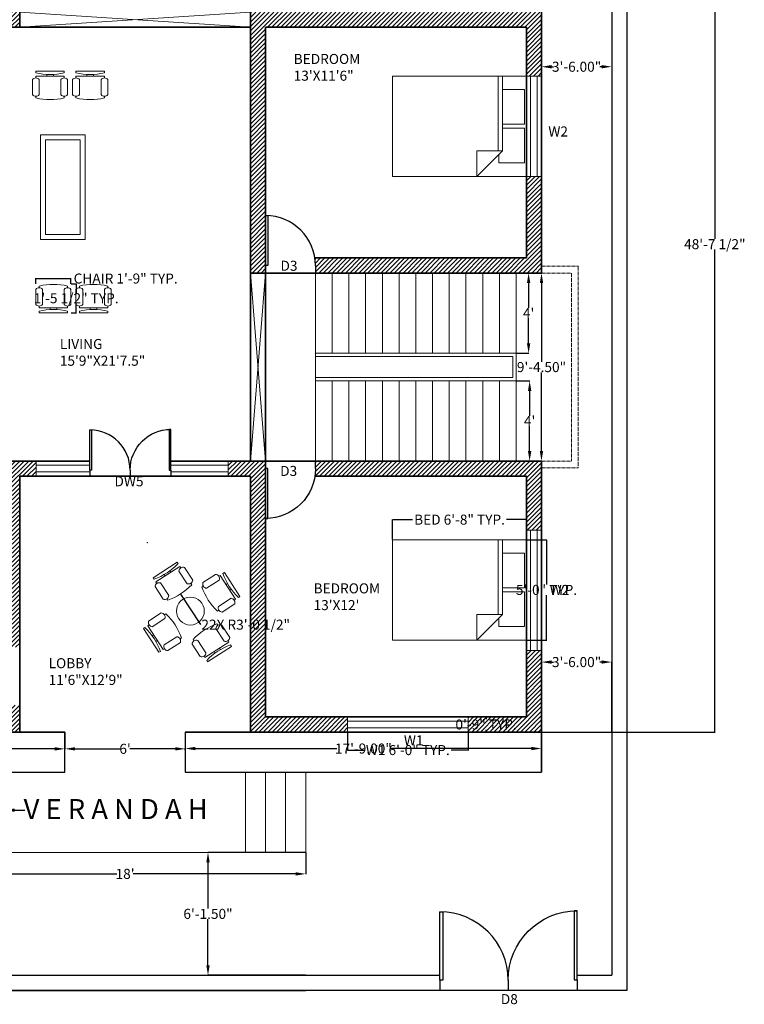
# Model space of a CAD drawing. Units: inches. Extents: x -57 to 1512, y -896 to 149.
# Tile 2 of 6: x 349 to 783, y -896 to -307. Entities that reach past the tile are written whole.
import ezdxf

# ---------------------------------------------------------------- set-up
doc = ezdxf.new("R2010")
doc.units = ezdxf.units.IN
doc.header["$MEASUREMENT"] = 0
doc.linetypes.add('ACAD_ISO02W100', pattern=[15, 12, -3])
doc.layers.get('Defpoints').update_dxf_attribs({"color": 9})
for name, color, linetype, lineweight in [('A-ANNO-DIMS', 2, 'Continuous', 18), ('A-ANNO-TEXT', 7, 'Continuous', 18), ('A-AREA-IDEN', 7, 'Continuous', 18), ('A-DOOR', 3, 'Continuous', 25), ('A-FLOR', 7, 'Continuous', 25), ('A-FLOR-OVHD', 8, 'ACAD_ISO02W100', 18), ('A-FLOR-STRS', 7, 'Continuous', 18), ('A-FURN', 8, 'Continuous', 18), ('A-GLAZ', 4, 'Continuous', 18), ('A-WALL', 7, 'Continuous', 35), ('A-WALL-OPEN', 7, 'Continuous', 18), ('A-WALL-PATT', 8, 'Continuous', 13), ('C-PROP', 7, 'Continuous', 25), ('L-SITE-GATE', 3, 'Continuous', 25)]:
    doc.layers.add(name, color=color, linetype=linetype, lineweight=lineweight)
doc.styles.get("Standard").update_dxf_attribs({"font": 'arial.ttf'})
doc.dimstyles.get("Standard").update_dxf_attribs({"dimtxt": 6, "dimasz": 0.18, "dimexe": 0.18, "dimexo": 0.0625, "dimgap": 0.09, "dimtad": 0, "dimtih": 1, "dimtoh": 1, "dimzin": 0, "dimdsep": 46, "dimlunit": 3, "dimtxsty": 'Standard', "dimcen": 0.09, "dimadec": 0, "dimazin": 0, "dimtfac": 1, "dimtofl": 0, "dimtmove": 0, "dimatfit": 3, "dimfxl": 1, "dimtolj": 1, "dimtzin": 0, "dimarcsym": 0})

# ---------------------------------------------------------------- blocks, each defined once
blk = doc.blocks.new('*U2')
for p, q in [((0, 0), (0, -6)), ((40, 0), (40, -6))]:
    blk.add_line(p, q)
blk.add_lwpolyline([(0, 0), (0, 40), (1.75, 40), (1.75, 0)], close=True)
blk.add_arc((0, 0), 40, 0, 90)
blk = doc.blocks.new('Bed - Queen')
for p, q in [((0, -80.00003), (0, 0)), ((0, 0), (59.99999, 0)), ((59.99999, 0), (59.99999, -80.00003)), ((7.99999, -1.2), (28.79998, -1.2)), ((7.99999, -14.4), (7.99999, -1.2)), ((28.79998, -1.2), (28.79998, -14.4)), ((31.19999, -1.2), (51.99999, -1.2)), ((31.19999, -14.4), (31.19999, -1.2)), ((51.99999, -1.2), (51.99999, -16.4)), ((0, -14.4), (44.8, -14.4)), ((44.8, -16.8), (0, -16.8)), ((59.99999, -29.6), (44.8, -14.4)), ((44.8, -14.4), (44.8, -29.6)), ((51.99999, -16.4), (46.79936, -16.4)), ((44.8, -29.6), (59.99999, -29.6)), ((59.99999, -80.00003), (0, -80.00003))]:
    blk.add_line(p, q)
blk = doc.blocks.new('Chair - Desk')
for p, q in [((-8.5, 0), (-8.5, -1)), ((-8.5, 0), (8.5, 0)), ((8.5, 0), (8.5, -1)), ((-10.5, -5), (-10.5, -14)), ((-8.5, -3), (-8.5, -4)), ((-8.5, -3), (8.5, -3)), ((-6.5, -14), (-6.5, -5)), ((-2, -3), (-2, -1.9355)), ((2, -1.9576), (2, -3)), ((6.5, -5), (6.5, -14)), ((8.5, -3), (8.5, -4)), ((10.5, -14), (10.5, -5)), ((-8.5, -15), (-8.5, -16)), ((8.5, -15), (8.5, -16))]:
    blk.add_line(p, q)
for centre, radius, start, end in [((-8.5, -6.5), 2.5, 36.8699, 143.1301), ((0, 34.625), 36.625, 256.5803, 283.4197), ((8.5, -6.5), 2.5, 36.8699, 143.1301), ((-8.5, -12.5), 2.5, 216.8699, 323.1301), ((0, 19.625), 36.625, 256.5803, 283.4197), ((8.5, -12.5), 2.5, 216.8699, 323.1301)]:
    blk.add_arc(centre, radius, start, end)
blk = doc.blocks.new('*D9')
at = {"layer": 'A-ANNO-DIMS', "color": 0, "lineweight": -2, "transparency": 16777216}
for p, q in [((661.3, -302.32), (661.3, -335.07)), ((703.3, -302.32), (703.3, -335.07)), ((667.3, -334.89), (668.41, -334.89)), ((697.3, -334.89), (696.18, -334.89))]:
    blk.add_line(p, q, dxfattribs=at)
at = {"layer": 'A-ANNO-DIMS', "color": 0, "transparency": 16777216}
for points in [[(667.3, -333.89), (667.3, -335.89), (661.3, -334.89)], [(697.3, -333.89), (697.3, -335.89), (703.3, -334.89)]]:
    blk.add_solid(points, dxfattribs=at)
at = {"layer": 'Defpoints', "color": 0, "transparency": 16777216}
for p in [(661.3, -302.26), (703.3, -302.26), (703.3, -334.89)]:
    blk.add_point(p, dxfattribs=at)
at = {"layer": 'A-ANNO-DIMS', "color": 0, "transparency": 16777216, "insert": (682.3, -334.89), "char_height": 6, "attachment_point": 5}
blk.add_mtext('\\A1;3\'-6.00"', dxfattribs=at)
blk = doc.blocks.new('*D10')
at = {"layer": 'A-ANNO-DIMS', "color": 0, "lineweight": -2, "transparency": 16777216}
for p, q in [((661.3, -732.7), (661.3, -690.75)), ((667.3, -690.93), (668.41, -690.93)), ((697.3, -690.93), (696.18, -690.93)), ((703.3, -732.7), (703.3, -690.75))]:
    blk.add_line(p, q, dxfattribs=at)
at = {"layer": 'A-ANNO-DIMS', "color": 0, "transparency": 16777216}
for points in [[(667.3, -689.93), (667.3, -691.93), (661.3, -690.93)], [(697.3, -689.93), (697.3, -691.93), (703.3, -690.93)]]:
    blk.add_solid(points, dxfattribs=at)
at = {"layer": 'Defpoints', "color": 0, "transparency": 16777216}
for p in [(703.3, -690.93), (661.3, -732.76), (703.3, -732.76)]:
    blk.add_point(p, dxfattribs=at)
at = {"layer": 'A-ANNO-DIMS', "color": 0, "transparency": 16777216, "insert": (682.3, -690.93), "char_height": 6, "attachment_point": 5}
blk.add_mtext('\\A1;3\'-6.00"', dxfattribs=at)
blk = doc.blocks.new('*D11')
at = {"layer": 'A-ANNO-DIMS', "color": 0, "lineweight": -2, "transparency": 16777216}
for p, q in [((448.3, -732.82), (448.3, -742.82)), ((661.3, -732.82), (661.3, -742.82)), ((454.3, -742.64), (538.86, -742.64)), ((655.3, -742.64), (570.74, -742.64))]:
    blk.add_line(p, q, dxfattribs=at)
at = {"layer": 'A-ANNO-DIMS', "color": 0, "transparency": 16777216}
for points in [[(454.3, -741.64), (454.3, -743.64), (448.3, -742.64)], [(655.3, -741.64), (655.3, -743.64), (661.3, -742.64)]]:
    blk.add_solid(points, dxfattribs=at)
at = {"layer": 'Defpoints', "color": 0, "transparency": 16777216}
for p in [(448.3, -732.76), (661.3, -732.76), (661.3, -742.64)]:
    blk.add_point(p, dxfattribs=at)
at = {"layer": 'A-ANNO-DIMS', "color": 0, "transparency": 16777216, "insert": (554.8, -742.64), "char_height": 6, "attachment_point": 5}
blk.add_mtext('\\A1;17\'-9.00"', dxfattribs=at)
blk = doc.blocks.new('*D12')
at = {"layer": 'A-ANNO-DIMS', "color": 0, "lineweight": -2, "transparency": 16777216}
for p, q in [((376.3, -743.58), (376.3, -742.64)), ((382.3, -742.82), (409.43, -742.82)), ((442.3, -742.82), (415.16, -742.82)), ((448.3, -743.58), (448.3, -742.64))]:
    blk.add_line(p, q, dxfattribs=at)
at = {"layer": 'A-ANNO-DIMS', "color": 0, "transparency": 16777216}
for points in [[(382.3, -741.82), (382.3, -743.82), (376.3, -742.82)], [(442.3, -741.82), (442.3, -743.82), (448.3, -742.82)]]:
    blk.add_solid(points, dxfattribs=at)
at = {"layer": 'Defpoints', "color": 0, "transparency": 16777216}
for p in [(376.3, -743.65), (448.3, -742.82), (448.3, -743.65)]:
    blk.add_point(p, dxfattribs=at)
at = {"layer": 'A-ANNO-DIMS', "color": 0, "transparency": 16777216, "insert": (412.3, -742.82), "char_height": 6, "attachment_point": 5}
blk.add_mtext("\\A1;6'", dxfattribs=at)
blk = doc.blocks.new('*D13')
at = {"layer": 'A-ANNO-DIMS', "color": 0, "lineweight": -2, "transparency": 16777216}
for p, q in [((163.3, -732.82), (163.3, -743.03)), ((376.3, -732.82), (376.3, -743.03)), ((169.3, -742.85), (253.86, -742.85)), ((370.3, -742.85), (285.74, -742.85))]:
    blk.add_line(p, q, dxfattribs=at)
at = {"layer": 'A-ANNO-DIMS', "color": 0, "transparency": 16777216}
for points in [[(169.3, -741.85), (169.3, -743.85), (163.3, -742.85)], [(370.3, -741.85), (370.3, -743.85), (376.3, -742.85)]]:
    blk.add_solid(points, dxfattribs=at)
at = {"layer": 'Defpoints', "color": 0, "transparency": 16777216}
for p in [(163.3, -732.76), (376.3, -732.76), (376.3, -742.85)]:
    blk.add_point(p, dxfattribs=at)
at = {"layer": 'A-ANNO-DIMS', "color": 0, "transparency": 16777216, "insert": (269.8, -742.85), "char_height": 6, "attachment_point": 5}
blk.add_mtext('\\A1;17\'-9.00"', dxfattribs=at)
blk = doc.blocks.new('*D14')
at = {"layer": 'A-ANNO-DIMS', "color": 0, "lineweight": -2, "transparency": 16777216}
for p, q in [((304.3, -804.82), (304.3, -817.78)), ((520.3, -804.82), (520.3, -817.78)), ((310.3, -817.6), (407.4, -817.6)), ((514.3, -817.6), (417.19, -817.6))]:
    blk.add_line(p, q, dxfattribs=at)
at = {"layer": 'A-ANNO-DIMS', "color": 0, "transparency": 16777216}
for points in [[(310.3, -816.6), (310.3, -818.6), (304.3, -817.6)], [(514.3, -816.6), (514.3, -818.6), (520.3, -817.6)]]:
    blk.add_solid(points, dxfattribs=at)
at = {"layer": 'Defpoints', "color": 0, "transparency": 16777216}
for p in [(304.3, -804.76), (520.3, -804.76), (520.3, -817.6)]:
    blk.add_point(p, dxfattribs=at)
at = {"layer": 'A-ANNO-DIMS', "color": 0, "transparency": 16777216, "insert": (412.3, -817.6), "char_height": 6, "attachment_point": 5}
blk.add_mtext("\\A1;18'", dxfattribs=at)
blk = doc.blocks.new('*D15')
at = {"layer": 'A-ANNO-DIMS', "color": 0, "lineweight": -2, "transparency": 16777216}
for p, q in [((328.3, -756.82), (328.3, -779.69)), ((340.3, -756.82), (340.3, -779.69)), ((322.3, -779.51), (316.3, -779.51)), ((346.3, -779.51), (352.3, -779.51))]:
    blk.add_line(p, q, dxfattribs=at)
at = {"layer": 'A-ANNO-DIMS', "color": 0, "transparency": 16777216}
for points in [[(322.3, -778.51), (322.3, -780.51), (328.3, -779.51)], [(346.3, -778.51), (346.3, -780.51), (340.3, -779.51)]]:
    blk.add_solid(points, dxfattribs=at)
at = {"layer": 'Defpoints', "color": 0, "transparency": 16777216}
for p in [(328.3, -756.76), (340.3, -756.76), (340.3, -779.51)]:
    blk.add_point(p, dxfattribs=at)
at = {"layer": 'A-ANNO-DIMS', "color": 0, "transparency": 16777216, "insert": (334.3, -779.51), "char_height": 6, "attachment_point": 5}
blk.add_mtext("\\A1;1'", dxfattribs=at)
blk = doc.blocks.new('*D16')
at = {"layer": 'A-ANNO-DIMS', "color": 0, "lineweight": -2, "transparency": 16777216}
for p, q in [((520.23, -804.76), (461.71, -804.76)), ((461.89, -810.76), (461.89, -838.36)), ((461.89, -872.26), (461.89, -844.66)), ((520.23, -878.26), (461.71, -878.26))]:
    blk.add_line(p, q, dxfattribs=at)
at = {"layer": 'A-ANNO-DIMS', "color": 0, "transparency": 16777216}
for points in [[(460.89, -810.76), (462.89, -810.76), (461.89, -804.76)], [(460.89, -872.26), (462.89, -872.26), (461.89, -878.26)]]:
    blk.add_solid(points, dxfattribs=at)
at = {"layer": 'Defpoints', "color": 0, "transparency": 16777216}
for p in [(520.3, -804.76), (461.89, -878.26), (520.3, -878.26)]:
    blk.add_point(p, dxfattribs=at)
at = {"layer": 'A-ANNO-DIMS', "color": 0, "transparency": 16777216, "insert": (461.89, -841.51), "char_height": 6, "attachment_point": 5}
blk.add_mtext('\\A1;6\'-1.50"', dxfattribs=at)
blk = doc.blocks.new('*D27')
at = {"layer": 'A-ANNO-DIMS', "color": 0, "lineweight": -2, "transparency": 16777216}
for p, q in [((646.2, -458.26), (653.79, -458.26)), ((653.61, -464.26), (653.61, -479.17)), ((653.61, -500.26), (653.61, -485.35)), ((646.2, -506.26), (653.79, -506.26))]:
    blk.add_line(p, q, dxfattribs=at)
at = {"layer": 'A-ANNO-DIMS', "color": 0, "transparency": 16777216}
for points in [[(652.61, -464.26), (654.61, -464.26), (653.61, -458.26)], [(652.61, -500.26), (654.61, -500.26), (653.61, -506.26)]]:
    blk.add_solid(points, dxfattribs=at)
at = {"layer": 'Defpoints', "color": 0, "transparency": 16777216}
for p in [(646.14, -458.26), (646.14, -506.26), (653.61, -506.26)]:
    blk.add_point(p, dxfattribs=at)
at = {"layer": 'A-ANNO-DIMS', "color": 0, "transparency": 16777216, "insert": (653.61, -482.26), "char_height": 6, "attachment_point": 5}
blk.add_mtext("\\A1;4'", dxfattribs=at)
blk = doc.blocks.new('*D28')
at = {"layer": 'A-ANNO-DIMS', "color": 0, "lineweight": -2, "transparency": 16777216}
for p, q in [((646.2, -522.76), (654.4, -522.76)), ((654.22, -528.76), (654.22, -543.67)), ((654.22, -564.76), (654.22, -549.85)), ((646.2, -570.76), (654.4, -570.76))]:
    blk.add_line(p, q, dxfattribs=at)
at = {"layer": 'A-ANNO-DIMS', "color": 0, "transparency": 16777216}
for points in [[(653.22, -528.76), (655.22, -528.76), (654.22, -522.76)], [(653.22, -564.76), (655.22, -564.76), (654.22, -570.76)]]:
    blk.add_solid(points, dxfattribs=at)
at = {"layer": 'Defpoints', "color": 0, "transparency": 16777216}
for p in [(646.14, -522.76), (646.14, -570.76), (654.22, -570.76)]:
    blk.add_point(p, dxfattribs=at)
at = {"layer": 'A-ANNO-DIMS', "color": 0, "transparency": 16777216, "insert": (654.22, -546.76), "char_height": 6, "attachment_point": 5}
blk.add_mtext("\\A1;4'", dxfattribs=at)
blk = doc.blocks.new('*D29')
at = {"layer": 'A-ANNO-DIMS', "color": 0, "lineweight": -2, "transparency": 16777216}
for p, q in [((661.36, -458.26), (661.48, -458.26)), ((661.3, -464.26), (661.3, -511.36)), ((661.3, -564.76), (661.3, -517.66)), ((661.36, -570.76), (661.48, -570.76))]:
    blk.add_line(p, q, dxfattribs=at)
at = {"layer": 'A-ANNO-DIMS', "color": 0, "transparency": 16777216}
for points in [[(660.3, -464.26), (662.3, -464.26), (661.3, -458.26)], [(660.3, -564.76), (662.3, -564.76), (661.3, -570.76)]]:
    blk.add_solid(points, dxfattribs=at)
at = {"layer": 'Defpoints', "color": 0, "transparency": 16777216}
for p in [(661.3, -458.26), (661.3, -570.76), (661.3, -570.76)]:
    blk.add_point(p, dxfattribs=at)
at = {"layer": 'A-ANNO-DIMS', "color": 0, "transparency": 16777216, "insert": (661.3, -514.51), "char_height": 6, "attachment_point": 5}
blk.add_mtext('\\A1;9\'-4.50"', dxfattribs=at)
blk = doc.blocks.new('WIN-72IN')
for p, q in [((0, 0), (0, 9)), ((0, 6.5), (72, 6.5)), ((72, 0), (72, 9)), ((0, 2.5), (72, 2.5))]:
    blk.add_line(p, q)
blk = doc.blocks.new('*D89')
at = {"layer": 'A-ANNO-DIMS', "color": 0, "lineweight": -2, "transparency": 16777216}
for p, q in [((358.93, -464.63), (358.93, -461.37)), ((359.11, -461.55), (379.75, -461.55)), ((379.93, -464.63), (379.93, -461.37)), ((379.93, -461.55), (380.11, -461.55))]:
    blk.add_line(p, q, dxfattribs=at)
at = {"layer": 'A-ANNO-DIMS', "color": 0, "transparency": 16777216}
for points in [[(359.11, -461.52), (359.11, -461.58), (358.93, -461.55)], [(379.75, -461.52), (379.75, -461.58), (379.93, -461.55)]]:
    blk.add_solid(points, dxfattribs=at)
at = {"layer": 'Defpoints', "color": 0, "transparency": 16777216}
for p in [(358.93, -464.7), (379.93, -461.55), (379.93, -464.7)]:
    blk.add_point(p, dxfattribs=at)
at = {"layer": 'A-ANNO-DIMS', "color": 0, "transparency": 16777216, "insert": (412.66, -461.55), "char_height": 6, "attachment_point": 5}
blk.add_mtext('\\A1;CHAIR 1\'-9" TYP.', dxfattribs=at)
blk = doc.blocks.new('*D90')
at = {"layer": 'A-ANNO-DIMS', "color": 0, "lineweight": -2, "transparency": 16777216}
for p, q in [((380, -464.7), (383.26, -464.7)), ((383.08, -464.88), (383.08, -470.17)), ((383.08, -481.85), (383.08, -476.56)), ((380, -482.03), (383.26, -482.03))]:
    blk.add_line(p, q, dxfattribs=at)
at = {"layer": 'A-ANNO-DIMS', "color": 0, "transparency": 16777216}
for points in [[(383.05, -464.88), (383.11, -464.88), (383.08, -464.7)], [(383.05, -481.85), (383.11, -481.85), (383.08, -482.03)]]:
    blk.add_solid(points, dxfattribs=at)
at = {"layer": 'Defpoints', "color": 0, "transparency": 16777216}
for p in [(379.93, -464.7), (379.93, -482.03), (383.08, -482.03)]:
    blk.add_point(p, dxfattribs=at)
at = {"layer": 'A-ANNO-DIMS', "color": 0, "transparency": 16777216, "insert": (383.08, -473.36), "char_height": 6, "attachment_point": 5}
blk.add_mtext('\\A1;1\'-5 1/2" TYP.', dxfattribs=at)
blk = doc.blocks.new('*D95')
at = {"layer": 'A-ANNO-DIMS', "color": 0, "lineweight": -2, "transparency": 16777216}
for p, q in [((572.3, -617.68), (572.3, -605.57)), ((572.48, -605.75), (584.27, -605.75)), ((652.12, -605.75), (640.32, -605.75)), ((652.3, -617.68), (652.3, -605.57))]:
    blk.add_line(p, q, dxfattribs=at)
at = {"layer": 'A-ANNO-DIMS', "color": 0, "transparency": 16777216}
for points in [[(572.48, -605.72), (572.48, -605.78), (572.3, -605.75)], [(652.12, -605.72), (652.12, -605.78), (652.3, -605.75)]]:
    blk.add_solid(points, dxfattribs=at)
at = {"layer": 'Defpoints', "color": 0, "transparency": 16777216}
for p in [(652.3, -605.75), (572.3, -617.75), (652.3, -617.75)]:
    blk.add_point(p, dxfattribs=at)
at = {"layer": 'A-ANNO-DIMS', "color": 0, "transparency": 16777216, "insert": (612.3, -605.75), "char_height": 6, "attachment_point": 5}
blk.add_mtext('\\A1;BED 6\'-8" TYP.', dxfattribs=at)
blk = doc.blocks.new('*D96')
at = {"layer": 'A-ANNO-DIMS', "color": 0, "lineweight": -2, "transparency": 16777216}
for p, q in [((652.36, -617.75), (664.48, -617.75)), ((664.3, -617.93), (664.3, -644.59)), ((664.3, -677.57), (664.3, -650.9)), ((652.36, -677.75), (664.48, -677.75))]:
    blk.add_line(p, q, dxfattribs=at)
at = {"layer": 'A-ANNO-DIMS', "color": 0, "transparency": 16777216}
for points in [[(664.27, -617.93), (664.33, -617.93), (664.3, -617.75)], [(664.27, -677.57), (664.33, -677.57), (664.3, -677.75)]]:
    blk.add_solid(points, dxfattribs=at)
at = {"layer": 'Defpoints', "color": 0, "transparency": 16777216}
for p in [(652.3, -617.75), (652.3, -677.75), (664.3, -677.75)]:
    blk.add_point(p, dxfattribs=at)
at = {"layer": 'A-ANNO-DIMS', "color": 0, "transparency": 16777216, "insert": (664.3, -647.75), "char_height": 6, "attachment_point": 5}
blk.add_mtext('\\A1;5\'-0" TYP.', dxfattribs=at)
blk = doc.blocks.new('*D97')
at = {"layer": 'A-ANNO-DIMS', "color": 0, "lineweight": -2, "transparency": 16777216}
for p, q in [((545.37, -732.82), (545.37, -743.74)), ((617.37, -732.82), (617.37, -743.74)), ((545.55, -743.56), (555.42, -743.56)), ((617.19, -743.56), (607.32, -743.56))]:
    blk.add_line(p, q, dxfattribs=at)
at = {"layer": 'A-ANNO-DIMS', "color": 0, "transparency": 16777216}
for points in [[(545.55, -743.53), (545.55, -743.59), (545.37, -743.56)], [(617.19, -743.53), (617.19, -743.59), (617.37, -743.56)]]:
    blk.add_solid(points, dxfattribs=at)
at = {"layer": 'Defpoints', "color": 0, "transparency": 16777216}
for p in [(545.37, -732.76), (617.37, -732.76), (545.37, -743.56)]:
    blk.add_point(p, dxfattribs=at)
at = {"layer": 'A-ANNO-DIMS', "color": 0, "transparency": 16777216, "insert": (581.37, -743.56), "char_height": 6, "attachment_point": 5}
blk.add_mtext('\\A1;W1 6\'-0" TYP.', dxfattribs=at)
blk = doc.blocks.new('*D98')
at = {"layer": 'A-ANNO-DIMS', "color": 0, "lineweight": -2, "transparency": 16777216}
for p, q in [((617.43, -723.76), (628.35, -723.76)), ((628.17, -723.94), (628.17, -725.11)), ((617.43, -732.76), (628.35, -732.76)), ((628.17, -732.58), (628.17, -731.41))]:
    blk.add_line(p, q, dxfattribs=at)
at = {"layer": 'A-ANNO-DIMS', "color": 0, "transparency": 16777216}
for points in [[(628.14, -723.94), (628.2, -723.94), (628.17, -723.76)], [(628.14, -732.58), (628.2, -732.58), (628.17, -732.76)]]:
    blk.add_solid(points, dxfattribs=at)
at = {"layer": 'Defpoints', "color": 0, "transparency": 16777216}
for p in [(617.37, -723.76), (617.37, -732.76), (628.17, -732.76)]:
    blk.add_point(p, dxfattribs=at)
at = {"layer": 'A-ANNO-DIMS', "color": 0, "transparency": 16777216, "insert": (628.17, -728.26), "char_height": 6, "attachment_point": 5}
blk.add_mtext('\\A1;0\'-9" TYP.', dxfattribs=at)
blk = doc.blocks.new('*D104')
at = {"layer": 'A-ANNO-DIMS', "color": 0, "lineweight": -2, "transparency": 16777216}
for p, q in [((631.36, -149.26), (765.13, -149.26)), ((764.95, -149.44), (764.95, -437.82)), ((764.95, -732.58), (764.95, -444.2)), ((661.36, -732.76), (765.13, -732.76))]:
    blk.add_line(p, q, dxfattribs=at)
at = {"layer": 'A-ANNO-DIMS', "color": 0, "transparency": 16777216}
for points in [[(764.92, -149.44), (764.98, -149.44), (764.95, -149.26)], [(764.92, -732.58), (764.98, -732.58), (764.95, -732.76)]]:
    blk.add_solid(points, dxfattribs=at)
at = {"layer": 'Defpoints', "color": 0, "transparency": 16777216}
for p in [(631.3, -149.26), (764.95, -149.26), (661.3, -732.76)]:
    blk.add_point(p, dxfattribs=at)
at = {"layer": 'A-ANNO-DIMS', "color": 0, "transparency": 16777216, "insert": (764.95, -441.01), "char_height": 6, "attachment_point": 5}
blk.add_mtext('\\A1;48\'-7 1/2"', dxfattribs=at)
blk = doc.blocks.new('*D109')
at = {"layer": 'A-ANNO-DIMS', "color": 0, "lineweight": -2, "transparency": 16777216}
for p, q in [((425.53, -619.4), (425.71, -619.4)), ((425.62, -619.49), (425.62, -619.31)), ((457.51, -668.56), (445.65, -650.28)), ((457.69, -668.56), (457.51, -668.56))]:
    blk.add_line(p, q, dxfattribs=at)
at = {"layer": 'A-ANNO-DIMS', "color": 0, "transparency": 16777216}
blk.add_solid([(445.67, -650.26), (445.62, -650.3), (445.55, -650.13)], dxfattribs=at)
at = {"layer": 'Defpoints', "color": 0, "transparency": 16777216}
for p in [(425.62, -619.4), (445.55, -650.13)]:
    blk.add_point(p, dxfattribs=at)
at = {"layer": 'A-ANNO-DIMS', "color": 0, "transparency": 16777216, "insert": (484.44, -668.56), "char_height": 6, "attachment_point": 5}
blk.add_mtext('\\A1;22X R3\'-0 1/2"', dxfattribs=at)

msp = doc.modelspace()

# ---------------------------------------------------------------- hatches: boundary and pattern name
at = {"layer": 'A-WALL-PATT'}
h = msp.add_hatch(dxfattribs=at)
h.set_pattern_fill('ANSI31', color=256, scale=15)
h.paths.add_polyline_path([(496.296, -570.76), (487.296, -570.76), (474.037, -570.76), (474.037, -579.76), (487.296, -579.76), (487.296, -732.76), (545.372, -732.76), (545.372, -723.76), (496.296, -723.76)])
h.paths.add_polyline_path([(661.296, -684.034), (652.296, -684.034), (652.296, -723.76), (617.372, -723.76), (617.372, -732.76), (661.296, -732.76)])
h.paths.add_polyline_path([(298.296, -570.76), (208.296, -570.76), (208.296, -575.26), (172.296, -575.26), (172.296, -534.76), (163.296, -534.76), (163.296, -604.062), (172.296, -604.062), (172.296, -579.76), (298.296, -579.76)])
h.paths.add_polyline_path([(172.296, -494.26), (163.296, -494.26), (163.296, -498.76), (172.296, -498.76)])
h.paths.add_polyline_path([(242.796, -494.26), (172.296, -494.26), (172.296, -498.76), (238.296, -498.76), (242.796, -498.76)])
h.paths.add_polyline_path([(242.796, -522.76), (238.296, -522.76), (238.296, -570.76), (242.796, -570.76)])
h.paths.add_polyline_path([(142.296, -405.989), (133.296, -405.989), (133.296, -458.26), (250.953, -458.26), (250.953, -452.508, -0.0212094), (251.091, -449.26), (142.296, -449.26)])
h.paths.add_polyline_path([(298.296, -311.26), (349.296, -311.26), (349.296, -302.26), (345.753, -302.26), (322.135, -302.26), (133.296, -302.26), (133.296, -345.989), (142.296, -345.989), (142.296, -311.26), (289.296, -311.26), (289.296, -458.26), (298.296, -458.26)])
h.paths.add_polyline_path([(172.296, -275.26), (163.296, -275.26), (163.296, -302.26), (172.296, -302.26)])
h.paths.add_polyline_path([(172.296, -158.26), (230.655, -158.26), (230.655, -149.26), (163.296, -149.26), (163.296, -215.26), (172.296, -215.26)])
h.paths.add_polyline_path([(378.235, -149.26), (266.655, -149.26), (266.655, -158.26), (378.235, -158.26)])
h.paths.add_polyline_path([(349.296, -158.26), (340.296, -158.26), (340.296, -279.28, -0.0583572), (345.753, -278.641), (349.296, -278.641)])
h.paths.add_polyline_path([(529.979, -149.26), (450.235, -149.26), (450.235, -158.26), (529.979, -158.26)])
h.paths.add_polyline_path([(496.296, -158.26), (487.296, -158.26), (487.296, -278.641), (490.839, -278.641, -0.0583572), (496.296, -279.28)])
h.paths.add_polyline_path([(631.296, -149.26), (589.979, -149.26), (589.979, -158.26), (622.296, -158.26), (622.296, -215.26), (631.296, -215.26)])
h.paths.add_polyline_path([(661.296, -302.26), (631.296, -302.26), (631.296, -275.26), (622.296, -275.26), (622.296, -302.26), (487.296, -302.26), (487.296, -458.26), (496.296, -458.26), (496.296, -453.783), (496.296, -423.936), (496.296, -311.26), (652.296, -311.26), (652.296, -340.453), (661.296, -340.453)])
h.paths.add_polyline_path([(349.296, -579.76), (359.066, -579.76), (359.066, -570.76), (340.296, -570.76), (340.296, -682.249, -0.0275619), (344.104, -682.039), (349.296, -682.039)])
h.paths.add_polyline_path([(172.296, -676.062), (163.296, -676.062), (163.296, -732.76), (200.083, -732.76), (200.083, -723.76), (172.296, -723.76)])
h.paths.add_polyline_path([(349.296, -716.654), (344.104, -716.654), (340.296, -716.654), (340.296, -723.76), (272.083, -723.76), (272.083, -732.76), (349.296, -732.76)])
h = msp.add_hatch(dxfattribs=at)
h.set_pattern_fill('ANSI31', color=256, scale=15)
h.paths.add_polyline_path([(661.296, -400.453), (652.296, -400.453), (652.296, -449.26), (652.296, -458.26), (661.296, -458.26)])
h.paths.add_polyline_path([(652.296, -449.26), (525.797, -449.26, -0.0380515), (526.142, -453.783), (526.142, -458.26), (652.296, -458.26)])
h.paths.add_polyline_path([(661.296, -570.76), (526.142, -570.76), (526.142, -575.236, -0.0380515), (525.797, -579.76), (652.296, -579.76), (652.296, -612.034), (661.296, -612.034)])

# ---------------------------------------------------------------- linework, layer by layer
at = {"layer": 'A-FLOR'}
for p, q in [((376.296, -756.76), (376.296, -732.76)), ((448.296, -732.76), (448.296, -756.76)), ((163.296, -756.76), (376.296, -756.76)), ((448.296, -756.76), (661.296, -756.76))]:
    msp.add_line(p, q, dxfattribs=at)
at = {"layer": 'A-FLOR-OVHD', "ltscale": 0.2}
for p, q in [((661.296, -454.26), (683.296, -454.26)), ((661.296, -458.26), (679.296, -458.26)), ((679.296, -458.26), (679.296, -570.76)), ((683.296, -454.26), (683.296, -574.76)), ((661.296, -570.76), (679.296, -570.76)), ((661.296, -574.76), (683.296, -574.76))]:
    msp.add_line(p, q, dxfattribs=at)
at = {"layer": 'A-FLOR-STRS'}
for p, q in [((526.142, -458.26), (526.142, -570.76)), ((536.142, -458.26), (536.142, -506.26)), ((546.142, -458.26), (546.142, -506.26)), ((556.142, -458.26), (556.142, -506.26)), ((566.142, -458.26), (566.142, -506.26)), ((576.142, -458.26), (576.142, -506.26)), ((586.142, -458.26), (586.142, -506.26)), ((596.142, -458.26), (596.142, -506.26)), ((606.142, -458.26), (606.142, -506.26)), ((616.142, -458.26), (616.142, -506.26)), ((626.142, -458.26), (626.142, -506.26)), ((636.142, -458.26), (636.142, -506.26)), ((646.142, -458.26), (646.142, -570.76)), ((526.142, -506.26), (646.142, -506.26)), ((526.142, -508.26), (644.142, -508.26)), ((644.142, -508.26), (644.142, -520.76)), ((526.142, -520.76), (644.142, -520.76)), ((526.142, -522.76), (646.142, -522.76)), ((536.142, -522.76), (536.142, -570.76)), ((546.142, -522.76), (546.142, -570.76)), ((556.142, -522.76), (556.142, -570.76)), ((566.142, -522.76), (566.142, -570.76)), ((576.142, -522.76), (576.142, -570.76)), ((586.142, -522.76), (586.142, -570.76)), ((596.142, -522.76), (596.142, -570.76)), ((606.142, -522.76), (606.142, -570.76)), ((616.142, -522.76), (616.142, -570.76)), ((626.142, -522.76), (626.142, -570.76)), ((636.142, -522.76), (636.142, -570.76)), ((484.296, -804.76), (484.296, -756.76)), ((496.296, -804.76), (496.296, -756.76)), ((508.296, -804.76), (508.296, -756.76)), ((520.296, -804.76), (520.296, -756.76)), ((304.296, -804.76), (520.296, -804.76))]:
    msp.add_line(p, q, dxfattribs=at)
at = {"layer": 'A-FURN'}
for points in [[(361.803, -375.651), (388.437, -375.651), (388.437, -438.191), (361.803, -438.191)], [(364.803, -378.651), (385.437, -378.651), (385.437, -435.191), (364.803, -435.191)]]:
    msp.add_lwpolyline(points, close=True, dxfattribs=at)
msp.add_circle((451.37, -660.447), 8.315, dxfattribs=at)
at = {"layer": 'A-GLAZ'}
for p, q in [((652.296, -340.453), (661.296, -340.453)), ((654.796, -340.453), (654.796, -400.453)), ((658.796, -340.453), (658.796, -400.453)), ((652.296, -400.453), (661.296, -400.453)), ((359.066, -579.76), (359.066, -570.76)), ((474.037, -579.76), (474.037, -570.76)), ((359.066, -573.26), (391.277, -573.26)), ((439.679, -573.26), (474.037, -573.26)), ((359.066, -577.26), (391.277, -577.26)), ((439.679, -577.26), (474.037, -577.26)), ((652.296, -612.034), (661.296, -612.034)), ((654.796, -612.034), (654.796, -684.034)), ((658.796, -612.034), (658.796, -684.034)), ((652.296, -684.034), (661.296, -684.034))]:
    msp.add_line(p, q, dxfattribs=at)
at = {"layer": 'A-WALL'}
for p, q in [((349.296, -158.26), (349.296, -311.26)), ((487.296, -302.26), (487.296, -570.76)), ((661.296, -302.26), (661.296, -458.26)), ((298.296, -311.26), (487.296, -311.26)), ((496.296, -311.26), (496.296, -723.76)), ((496.296, -311.26), (652.296, -311.26)), ((652.296, -311.26), (652.296, -449.26)), ((525.797, -449.26), (652.296, -449.26)), ((487.296, -458.26), (661.296, -458.26)), ((208.296, -570.76), (391.277, -570.76)), ((439.679, -570.76), (661.296, -570.76)), ((496.296, -570.76), (487.296, -570.76)), ((661.296, -570.76), (661.296, -756.76)), ((349.296, -579.76), (349.296, -732.76)), ((349.296, -579.76), (487.296, -579.76)), ((487.296, -579.76), (487.296, -732.76)), ((525.797, -579.76), (652.296, -579.76)), ((652.296, -579.76), (652.296, -723.76)), ((496.296, -723.76), (652.296, -723.76)), ((163.296, -732.76), (376.296, -732.76)), ((448.296, -732.76), (661.296, -732.76))]:
    msp.add_line(p, q, dxfattribs=at)
at = {"layer": 'A-WALL-OPEN'}
for p, q in [((349.296, -302.26), (487.296, -311.26)), ((349.296, -311.26), (487.296, -302.26)), ((487.296, -458.26), (496.296, -570.76)), ((487.296, -570.76), (496.296, -458.26))]:
    msp.add_line(p, q, dxfattribs=at)
at = {"layer": 'C-PROP'}
for p, q in [((712.296, 24.74), (712.296, -887.26)), ((703.296, -302.26), (703.296, -458.26)), ((703.296, -458.26), (703.296, -878.26)), ((198.4, -878.26), (600.465, -878.26)), ((641.223, -878.26), (641.419, -878.26)), ((641.223, -878.26), (641.419, -878.26)), ((682.647, -878.26), (703.296, -878.26)), ((712.296, -887.26), (7.296, -887.26)), ((304.296, -887.26), (520.296, -887.26))]:
    msp.add_line(p, q, dxfattribs=at)

# ---------------------------------------------------------------- block references
at = {"layer": 'A-DOOR'}
for p, xscale, yscale, zscale in [((496.296, -453.783), 0.7461532224003351, 0.7461532224003351, 0.7461532224003351), ((391.277, -576.15), 0.6016115000971808, 0.6016115000971808, 0.6016115000971808), ((391.277, -576.15), 0.6016115000971808, 0.6016115000971808, 0.6016115000971808), ((439.679, -576.109), -0.6084364823532742, 0.6084364823532742, 0.6084364823532742), ((439.679, -576.109), -0.6084364823532742, 0.6084364823532742, 0.6084364823532742)]:
    msp.add_blockref('*U2', p, dxfattribs=dict(at, xscale=xscale, yscale=yscale, zscale=zscale))
at = {"layer": 'A-DOOR', "xscale": -0.7461532224003351, "yscale": 0.7461532224003351, "zscale": 0.7461532224003351, "rotation": 180}
msp.add_blockref('*U2', (496.296, -575.236), dxfattribs=at)
at = {"layer": 'A-FURN'}
for p in [(367.434, -337.584), (391.461, -337.584)]:
    msp.add_blockref('Chair - Desk', p, dxfattribs=at)
for name, p, rotation in [('Bed - Queen', (652.296, -340.453), 270), ('Bed - Queen', (652.296, -617.746), 270), ('Chair - Desk', (436.298, -635.865), 32.96667636562534), ('Chair - Desk', (476.326, -644.588), 302.9666763656253), ('Chair - Desk', (427.932, -677.972), 122.9666763656253), ('Chair - Desk', (468.813, -686.164), 212.9666763656253)]:
    msp.add_blockref(name, p, dxfattribs=dict(at, rotation=rotation))
at = {"layer": 'A-FURN', "xscale": -1, "rotation": 180}
for p in [(369.434, -482.03), (393.461, -482.03)]:
    msp.add_blockref('Chair - Desk', p, dxfattribs=at)
at = {"layer": 'A-GLAZ', "rotation": 180}
msp.add_blockref('WIN-72IN', (617.372, -723.759), dxfattribs=at)
at = {"layer": 'L-SITE-GATE'}
for p, xscale, yscale, zscale in [((600.465, -881.131), 1.021473734565475, 1.021473734565475, 1.021473734565475), ((682.647, -881.061), -1.033061844354514, 1.033061844354514, 1.033061844354514)]:
    msp.add_blockref('*U2', p, dxfattribs=dict(at, xscale=xscale, yscale=yscale, zscale=zscale))

# ---------------------------------------------------------------- texts
at = {"layer": 'A-ANNO-TEXT', "char_height": 6, "attachment_point": 1}
for s, heights, insert in [('W2', [0], (665.418, -370.629)), ('D3', [6.131], (505.231, -450.924)), ('D3', [6.131], (505.044, -573.629)), ('DW5', [6.131], (405.98, -579.817)), ('W2', [0], (666.241, -644.804)), ('W1', [0], (579.036, -734.75)), ('D8', [6.131], (636.991, -889.499))]:
    msp.add_mtext_dynamic_manual_height_columns(s, width=173.83392, gutter_width=1, heights=heights, dxfattribs=dict(at, insert=insert))
at = {"layer": 'A-AREA-IDEN', "attachment_point": 1}
for s, insert, char_height in [('BEDROOM\\P13\'X11\'6"', (513.129, -327.246), 6), ('LIVING\\P15\'9"X21\'7.5"', (373.292, -497.721), 6), ("BEDROOM\\P13'X12'", (525.009, -643.848), 6), ('LOBBY\\P11\'6"X12\'9"', (366.597, -688.597), 6), ('V E R A N D A H', (351.661, -772.854), 12)]:
    msp.add_mtext_dynamic_manual_height_columns(s, width=160.11736, gutter_width=1, heights=[0], dxfattribs=dict(at, insert=insert, char_height=char_height))

# ---------------------------------------------------------------- dimensions: what is measured, and where the dimension line sits
at = {"layer": 'A-ANNO-DIMS'}
for base, p1, p2, override, picture, middle in [((764.946, -149.26), (661.296, -732.76), (631.296, -149.26), {"dimdec": 1, "dimlfac": 1, "dimrnd": 0, "dimzin": 1, "dimdsep": 46, "dimlunit": 4, "dimfrac": 2}, '*D104', (764.946, -441.01)), ((653.606, -506.26), (646.142, -458.26), (646.142, -506.26), {"dimasz": 6, "dimclrd": 0, "dimclre": 0, "dimclrt": 0}, '*D27', (653.606, -482.26)), ((661.296, -570.76), (661.296, -458.26), (661.296, -570.76), {"dimasz": 6, "dimclrd": 0, "dimclre": 0, "dimclrt": 0}, '*D29', (661.296, -514.51)), ((654.218, -570.76), (646.142, -522.76), (646.142, -570.76), {"dimasz": 6, "dimclrd": 0, "dimclre": 0, "dimclrt": 0}, '*D28', (654.218, -546.76)), ((461.895, -878.26), (520.296, -804.76), (520.296, -878.26), {"dimasz": 6, "dimclrd": 0, "dimclre": 0, "dimclrt": 0}, '*D16', (461.895, -841.51))]:
    dim = msp.add_linear_dim(base=base, p1=p1, p2=p2, angle=90, dimstyle='Standard', override=override, dxfattribs=at)
    dim.commit()
    dim.dimension.update_dxf_attribs({"geometry": picture, "text_midpoint": middle})
for base, p1, p2, picture, middle in [((703.296, -334.886), (661.296, -302.26), (703.296, -302.26), '*D9', (682.296, -334.886)), ((703.296, -690.934), (661.296, -732.76), (703.296, -732.76), '*D10', (682.296, -690.934)), ((376.296, -742.845), (163.296, -732.76), (376.296, -732.76), '*D13', (269.796, -742.845)), ((661.296, -742.635), (448.296, -732.76), (661.296, -732.76), '*D11', (554.796, -742.635)), ((448.296, -742.815), (376.296, -743.646), (448.296, -743.646), '*D12', (412.296, -742.815)), ((340.296, -779.512), (328.296, -756.76), (340.296, -756.76), '*D15', (334.296, -779.512)), ((520.296, -817.601), (304.296, -804.76), (520.296, -804.76), '*D14', (412.296, -817.601))]:
    dim = msp.add_linear_dim(base=base, p1=p1, p2=p2, dimstyle='Standard', override={"dimasz": 6, "dimclrd": 0, "dimclre": 0, "dimclrt": 0}, dxfattribs=at)
    dim.commit()
    dim.dimension.update_dxf_attribs({"geometry": picture, "text_midpoint": middle})
for base, p1, p2, text, picture, middle in [((379.934, -461.547), (358.934, -464.697), (379.934, -464.697), 'CHAIR <> TYP.', '*D89', (412.66, -461.547)), ((652.296, -605.746), (572.296, -617.746), (652.296, -617.746), 'BED <> TYP.', '*D95', (612.296, -605.746))]:
    dim = msp.add_linear_dim(base=base, p1=p1, p2=p2, text=text, dimstyle='Standard', override={"dimdec": 1, "dimlfac": 1, "dimrnd": 0, "dimzin": 1, "dimdsep": 46, "dimlunit": 4, "dimfrac": 2}, dxfattribs=at)
    dim.commit()
    dim.dimension.update_dxf_attribs({"geometry": picture, "text_midpoint": middle})
for base, p1, p2, angle, text, picture, middle in [((383.084, -482.03), (379.934, -464.697), (379.934, -482.03), 270, '<> TYP.', '*D90', (383.084, -473.364)), ((664.296, -677.746), (652.296, -617.746), (652.296, -677.746), 270, '<> TYP.', '*D96', (664.296, -647.746)), ((628.172, -732.76), (617.372, -723.76), (617.372, -732.76), 270, '<> TYP.', '*D98', (628.172, -728.26)), ((545.372, -743.56), (617.372, -732.76), (545.372, -732.76), 180, 'W1 <> TYP.', '*D97', (581.372, -743.56))]:
    dim = msp.add_linear_dim(base=base, p1=p1, p2=p2, angle=angle, text=text, dimstyle='Standard', override={"dimdec": 1, "dimlfac": 1, "dimrnd": 0, "dimzin": 1, "dimdsep": 46, "dimlunit": 4, "dimfrac": 2}, dxfattribs=at)
    dim.commit()
    dim.dimension.update_dxf_attribs({"geometry": picture, "text_midpoint": middle})
dim = msp.add_radius_dim(center=(425.619, -619.4), mpoint=(445.549, -650.128), text='22X <>', dimstyle='Standard', override={"dimdec": 1, "dimlfac": 1, "dimrnd": 0, "dimzin": 1, "dimdsep": 46, "dimlunit": 4, "dimfrac": 2}, dxfattribs=at)
dim.commit()
dim.dimension.update_dxf_attribs({"geometry": '*D109', "text_midpoint": (484.441, -668.565), "dimtype": 164})

doc.saveas('drawing.dxf')
